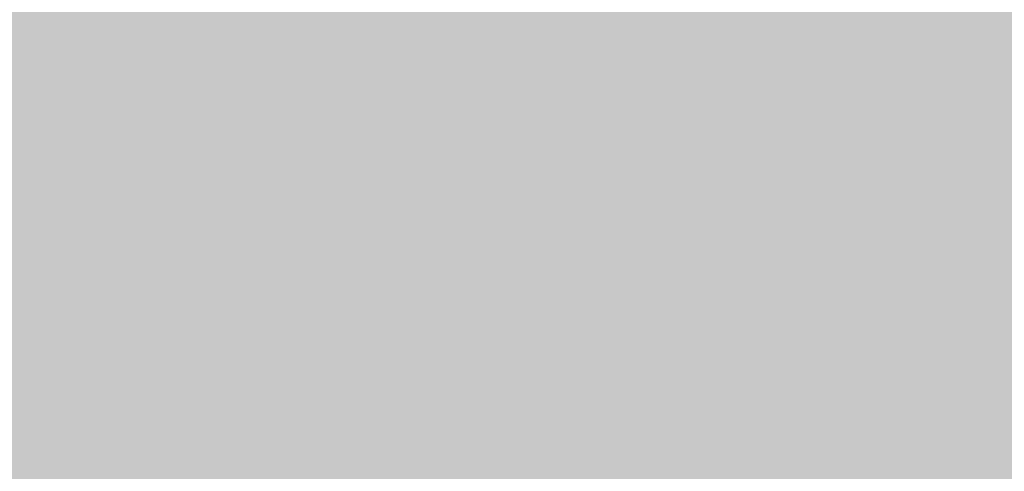
# Model space of a CAD drawing. Units: inches. Extents: x 2696 to 3240, y 1564 to 2310.
# Tile 68 of 76: x 3144.264 to 3152.299, y 2070.762 to 2074.447. Entities that reach past the tile are written whole.
import ezdxf

# ---------------------------------------------------------------- set-up
doc = ezdxf.new("R2010")
doc.units = ezdxf.units.IN
doc.layers.add('A-ANNO-DIMS', color=3, linetype='Continuous', lineweight=18)
doc.layers.add('A-WALL-PATT', color=9, linetype='Continuous', lineweight=13)
doc.styles.add('TIMES NEW', font='times.ttf')
doc.dimstyles.new('Siddhuu', dxfattribs={"dimtxt": 6, "dimasz": 2.5, "dimexe": 1.25, "dimexo": 0.625, "dimtad": 1, "dimdec": 1, "dimlunit": 4, "dimtxsty": 'TIMES NEW', "dimcen": 2.5, "dimclrd": 256, "dimclre": 1, "dimclrt": 7, "dimadec": 0, "dimazin": 0, "dimtfac": 1, "dimtdec": 1, "dimtmove": 0, "dimatfit": 3, "dimfxl": 1, "dimtolj": 1, "dimlwd": -1, "dimarcsym": 0})

# ---------------------------------------------------------------- blocks, each defined once
blk = doc.blocks.new('*D54')
at = {"layer": 'A-ANNO-DIMS', "color": 1, "lineweight": -2, "transparency": 16777216}
for p, q in [((3124.6114, 1893.8261), (3124.6114, 2298.4511)), ((3136.6114, 1893.8261), (3136.6114, 2298.4511))]:
    blk.add_line(p, q, dxfattribs=at)
at = {"layer": 'A-ANNO-DIMS', "transparency": 16777216}
for p, q in [((3127.1114, 2297.2011), (3134.1114, 2297.2011)), ((3136.6114, 2297.2011), (3155.7572, 2297.2011))]:
    blk.add_line(p, q, dxfattribs=at)
for points in [[(3127.1114, 2297.6178), (3127.1114, 2296.7844), (3124.6114, 2297.2011)], [(3134.1114, 2297.6178), (3134.1114, 2296.7844), (3136.6114, 2297.2011)]]:
    blk.add_solid(points, dxfattribs=at)
at = {"layer": 'Defpoints', "color": 0, "transparency": 16777216}
for p in [(3136.6114, 2297.2011), (3124.6114, 1893.2011), (3136.6114, 1893.2011)]:
    blk.add_point(p, dxfattribs=at)
at = {"layer": 'A-ANNO-DIMS', "color": 7, "transparency": 16777216, "insert": (3147.4343, 2300.878), "char_height": 6, "attachment_point": 5, "style": 'TIMES NEW'}
blk.add_mtext('\\A1;1\'-0"', dxfattribs=at)

msp = doc.modelspace()

# ---------------------------------------------------------------- hatches: boundary and pattern name
at = {"layer": 'A-WALL-PATT', "transparency": 33554556}
h = msp.add_hatch(color=256, dxfattribs=at)
h.dxf.hatch_style = 1
h.paths.add_polyline_path([(2879.1114, 2253.2011), (2905.9101, 2253.2011), (2905.9101, 2262.2011), (2841.889, 2262.2011), (2841.889, 2253.2011), (2870.1114, 2253.2011), (2870.1114, 2176.6011), (2965.7088, 2176.6011), (2965.7088, 2206.7011), (2973.5828, 2206.7011), (2973.5828, 2215.7011), (2965.7088, 2215.7011), (2965.7088, 2262.2011), (2929.9101, 2262.2011), (2929.9101, 2253.2011), (2956.7088, 2253.2011), (2956.7088, 2185.6011), (2879.1114, 2185.6011)])
h.paths.add_polyline_path([(2782.8338, 2262.2011), (2745.6114, 2262.2011), (2745.6114, 2228.7287), (2754.6114, 2228.7287), (2754.6114, 2253.2011), (2782.8338, 2253.2011)])
h.paths.add_polyline_path([(2754.6114, 2136.2011), (2965.7088, 2136.2011), (2965.7088, 2145.2011), (2879.1114, 2145.2011), (2879.1114, 2147.0735), (2877.3397, 2147.0735), (2870.1114, 2147.0735), (2870.1114, 2145.2011), (2754.6114, 2145.2011), (2754.6114, 2169.6735), (2745.6114, 2169.6735), (2745.6114, 2000.2011), (2754.6114, 2000.2011), (2754.6114, 2019.2011), (2849.0828, 2019.2011), (2849.0828, 2023.7011), (2841.2088, 2023.7011), (2841.2088, 2051.8271), (2836.7088, 2051.8271), (2836.7088, 2023.7011), (2754.6114, 2023.7011), (2754.6114, 2091.2011), (2836.7088, 2091.2011), (2836.7088, 2087.8271), (2841.2088, 2087.8271), (2841.2088, 2095.7011), (2754.6114, 2095.7011)])
h.paths.add_polyline_path([(2965.7088, 2136.2011), (2956.7088, 2136.2011), (2956.7088, 2023.7011), (2885.0828, 2023.7011), (2885.0828, 2019.2011), (2956.7088, 2019.2011), (2956.7088, 1950.5751), (2965.7088, 1950.5751), (2965.7088, 1980.2011), (2973.5828, 1980.2011), (2973.5828, 1989.2011), (2965.7088, 1989.2011)])
h.paths.add_polyline_path([(2754.6114, 1906.7011), (2880.2088, 1906.7011), (2884.7088, 1906.7011), (2956.7088, 1906.7011), (2956.7088, 1792.7011), (2944.7088, 1792.7011), (2944.7088, 1783.7011), (2956.7088, 1783.7011), (2956.7088, 1740.2011), (2884.7088, 1740.2011), (2884.7088, 1783.7011), (2896.7088, 1783.7011), (2896.7088, 1792.7011), (2884.7088, 1792.7011), (2884.7088, 1846.7011), (2880.2088, 1846.7011), (2880.2088, 1740.2011), (2754.6114, 1740.2011), (2754.6114, 1777.2011), (2745.6114, 1777.2011), (2745.6114, 1692.7011), (2754.6114, 1692.7011), (2754.6114, 1731.2011), (2956.7088, 1731.2011), (2956.7088, 1723.3271), (2965.7088, 1723.3271), (2965.7088, 1884.2011), (2973.5828, 1884.2011), (2973.5828, 1893.2011), (2965.7088, 1893.2011), (2965.7088, 1914.5751), (2956.7088, 1914.5751), (2956.7088, 1911.2011), (2754.6114, 1911.2011), (2754.6114, 1930.2011), (2745.6114, 1930.2011), (2745.6114, 1817.2011), (2754.6114, 1817.2011), (2754.6114, 1854.2011), (2826.6114, 1854.2011), (2826.6114, 1868.8271), (2822.1114, 1868.8271), (2822.1114, 1858.7011), (2754.6114, 1858.7011)])
h.paths.add_polyline_path([(2965.7088, 1656.2011), (3008.2374, 1656.2011), (3008.2374, 1665.2011), (2965.7088, 1665.2011), (2965.7088, 1693.3271), (2956.7088, 1693.3271), (2956.7088, 1686.2011), (2934.5828, 1686.2011), (2934.5828, 1681.7011), (2956.7088, 1681.7011), (2956.7088, 1614.2011), (2896.7088, 1614.2011), (2896.7088, 1681.7011), (2904.5828, 1681.7011), (2904.5828, 1686.2011), (2892.2088, 1686.2011), (2892.2088, 1614.2011), (2858.4101, 1614.2011), (2858.4101, 1605.2011), (2965.7088, 1605.2011)])
h.paths.add_polyline_path([(2788.4101, 1614.2011), (2754.6114, 1614.2011), (2754.6114, 1652.7011), (2745.6114, 1652.7011), (2745.6114, 1605.2011), (2788.4101, 1605.2011)])
h.paths.add_polyline_path([(3199.6114, 1633.0476), (3190.6114, 1633.0476), (3190.6114, 1614.2011), (3082.6114, 1614.2011), (3082.6114, 1665.2011), (3070.2374, 1665.2011), (3070.2374, 1656.2011), (3078.1114, 1656.2011), (3078.1114, 1605.2011), (3199.6114, 1605.2011)])
h.paths.add_polyline_path([(3199.6114, 1702.0476), (3190.6114, 1702.0476), (3190.6114, 1699.7011), (3106.6114, 1699.7011), (3106.6114, 1747.7011), (3190.6114, 1747.7011), (3190.6114, 1752.2011), (3082.6114, 1752.2011), (3082.6114, 1760.0751), (3078.1114, 1760.0751), (3078.1114, 1747.7011), (3102.1114, 1747.7011), (3102.1114, 1699.7011), (3078.1114, 1699.7011), (3078.1114, 1695.2011), (3190.6114, 1695.2011), (3190.6114, 1676.3546), (3199.6114, 1676.3546)])
h.paths.add_polyline_path([(3199.6114, 1783.2011), (3190.6114, 1783.2011), (3190.6114, 1745.3546), (3199.6114, 1745.3546)])
h.paths.add_polyline_path([(3082.6114, 1884.2011), (3190.6114, 1884.2011), (3190.6114, 1853.2011), (3199.6114, 1853.2011), (3199.6114, 1901.7011), (3190.6114, 1901.7011), (3190.6114, 1893.2011), (3005.5828, 1893.2011), (3005.5828, 1891.2811), (3005.5828, 1884.2011), (3078.1114, 1884.2011), (3078.1114, 1792.0751), (3082.6114, 1792.0751)])
h.paths.add_polyline_path([(3199.6114, 1994.7011), (3190.6114, 1994.7011), (3190.6114, 1989.2011), (3073.7088, 1989.2011), (3073.7088, 2034.2011), (3069.2088, 2034.2011), (3069.2088, 1989.2011), (3005.5828, 1989.2011), (3005.5828, 1980.2011), (3190.6114, 1980.2011), (3190.6114, 1971.7011), (3199.6114, 1971.7011)])
h.paths.add_polyline_path([(3199.6114, 2155.2011), (3190.6114, 2155.2011), (3190.6114, 2064.7011), (3199.6114, 2064.7011)])
h.paths.add_polyline_path([(3190.6114, 2074.7011), (3106.6114, 2074.7011), (3106.6114, 2122.7011), (3190.6114, 2122.7011), (3190.6114, 2127.2011), (3082.7088, 2127.2011), (3082.7088, 2135.0751), (3073.7088, 2135.0751), (3073.7088, 2122.7011), (3102.1114, 2122.7011), (3102.1114, 2074.7011), (3069.2088, 2074.7011), (3069.2088, 2070.2011), (3190.6114, 2070.2011)])
h.paths.add_polyline_path([(3082.7088, 2253.2011), (3190.6114, 2253.2011), (3190.6114, 2225.2011), (3199.6114, 2225.2011), (3199.6114, 2262.2011), (3073.7088, 2262.2011), (3073.7088, 2215.7011), (3035.5828, 2215.7011), (3035.5828, 2206.7011), (3073.7088, 2206.7011), (3073.7088, 2171.0751), (3082.7088, 2171.0751)])

# ---------------------------------------------------------------- dimensions: what is measured, and where the dimension line sits
at = {"layer": 'A-ANNO-DIMS'}
dim = msp.add_linear_dim(base=(3136.6114, 2297.2011), p1=(3124.6114, 1893.2011), p2=(3136.6114, 1893.2011), dimstyle='Siddhuu', override={"dimdec": 1, "dimlfac": 1, "dimrnd": 0, "dimzin": 1, "dimdsep": 46, "dimlunit": 4, "dimfrac": 2}, dxfattribs=at)
dim.commit()
dim.dimension.update_dxf_attribs({"geometry": '*D54', "text_midpoint": (3147.4343, 2300.878)})

doc.saveas('drawing.dxf')
